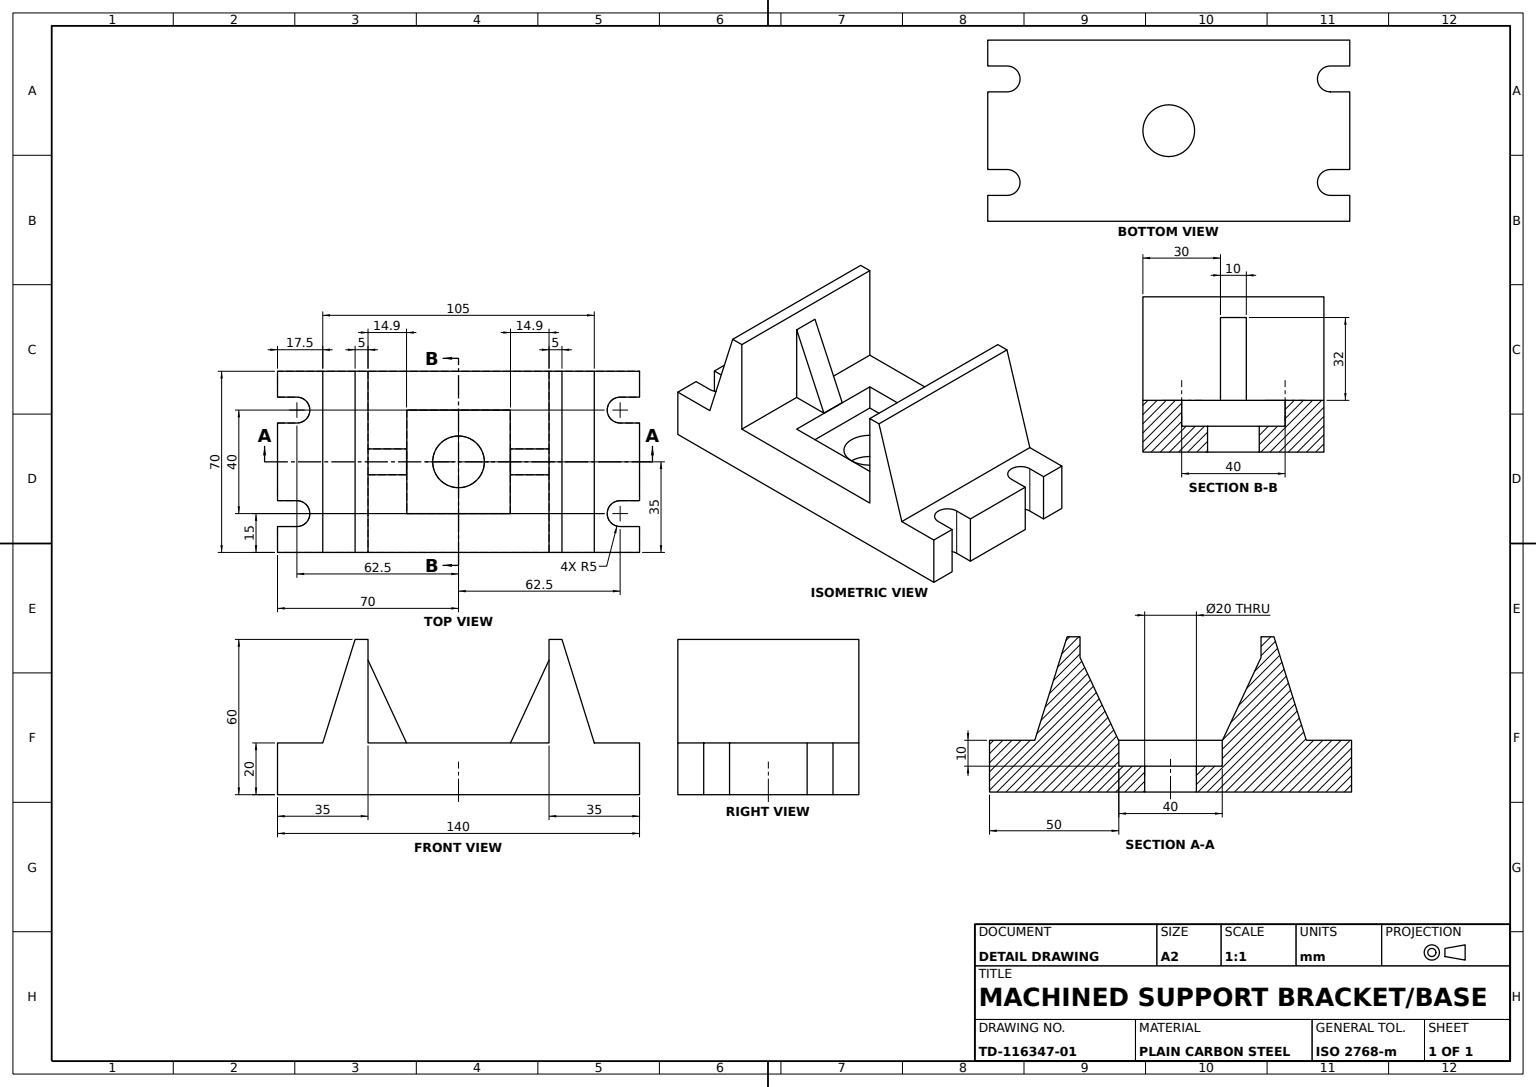
SolidWorks part; units mm, degrees
material "Plain Carbon Steel"
ref_plane "Front Plane" through (0, 0, 0) normal (0, 0, 1) x (1, 0, 0)
ref_plane "Top Plane" through (0, 0, 0) normal (0, 1, 0) x (1, 0, 0)
ref_plane "Right Plane" through (0, 0, 0) normal (1, 0, 0) x (0, 0, -1)
sketch "Base Plate Sketch" plane through (0, 0, 0) normal (0, 1, 0) x (1, 0, 0)
  line L0 (-70, 25) -> (-62.5, 25)
  line L1 (-70, 35) -> (70, 35)
  line L2 (-70, 35) -> (-70, 25)
  line L3 (-70, -35) -> (70, -35)
  line L4 (70, 35) -> (70, 25)
  line L5 (-70, 35) -> (70, -35) construction
  line L6 (-70, -35) -> (70, 35) construction
  line L8 (70, 15) -> (62.5, 15)
  line L9 (-70, -15) -> (-62.5, -15)
  line L11 (70, -25) -> (62.5, -25)
  line L12 (-70, 15) -> (-70, -15)
  line L13 (62.5, 25) -> (70, 25)
  line L14 (-62.5, 15) -> (-70, 15)
  line L15 (70, 15) -> (70, -15)
  line L16 (-70, -25) -> (-70, -35)
  line L17 (62.5, -15) -> (70, -15)
  line L18 (-62.5, -25) -> (-70, -25)
  line L19 (70, -25) -> (70, -35)
  arc A0 (-62.5, -25) -> (-62.5, -15) centre (-62.5, -20) ccw
  arc A1 (-62.5, 15) -> (-62.5, 25) centre (-62.5, 20) ccw
  arc A2 (62.5, 25) -> (62.5, 15) centre (62.5, 20) ccw
  arc A3 (62.5, -15) -> (62.5, -25) centre (62.5, -20) ccw
  point P8 (0, 0)
  dimension "D1" = 20
  dimension "D11" = 10
  dimension "D12" = 10
  dimension "D13" = 10
  dimension "D14" = 10
  dimension "D2" = 20
  dimension "D3" = 20
  dimension "D4" = 20
  dimension "D5" = 62.5
  dimension "D6" = 62.5
  dimension "D7" = 62.5
  dimension "D8" = 62.5
  dimension "D9" = 70
  dimension "D10" = 140
extrude "Base Plate 140x70x20" add sketch "Base Plate Sketch" along normal blind 20
sketch "Centre Hole Sketch" plane through (0, 20, 0) normal (0, 1, 0) x (1, 0, 0)
  circle A0 centre (0, 0) radius 10
  dimension "D1" = 20
extrude "Centre Hole Ø20" cut sketch "Centre Hole Sketch" against normal blind 20
sketch "Centre Pocket Sketch" plane through (0, 20, 0) normal (0, 1, 0) x (1, 0, 0)
  line L1 (-20, 20) -> (20, 20)
  line L2 (-20, 20) -> (-20, -20)
  line L3 (-20, -20) -> (20, -20)
  line L4 (20, 20) -> (20, -20)
  line L5 (-20, 20) -> (20, -20) construction
  line L6 (-20, -20) -> (20, 20) construction
  point P0 (0, 0)
  dimension "D1" = 40
extrude "Centre Pocket 40x40x10" cut sketch "Centre Pocket Sketch" against normal blind 10
sketch "V-Block Uprights Sketch" plane through (0, 0, 35) normal (0, 0, 1) x (1, 0, 0)
  line L0 (-52.5, 20) -> (-35, 20)
  line L1 (-70, 20) -> (70, 20) construction
  line L3 (-70, 20) -> (-70, 0) construction
  line L4 (70, 20) -> (70, 0) construction
  line L6 (35, 20) -> (52.5, 20)
  line L7 (-35, 60) -> (-40, 60)
  line L8 (-40, 60) -> (-52.5, 20)
  line L9 (-35, 20) -> (-35, 60)
  line L10 (35, 60) -> (35, 20)
  line L11 (35, 20) -> (52.5, 20)
  line L12 (35, 60) -> (40, 60)
  line L13 (40, 60) -> (52.5, 20)
  line L14 (35, 20) -> (52.5, 20)
  point P5 (0, 20)
  line M9 (70, 20) -> (-70, 20)
  dimension "D1" = 105
  dimension "D2" = 17.5
  dimension "D3" = 17.5
  dimension "D4" = 70
  dimension "D5" = 40
  dimension "D6" = 17.5
  dimension "D7" = 5
  dimension "D8" = 17.5
  dimension "D9" = 5
extrude "V-Block Uprights" add sketch "V-Block Uprights Sketch" against normal blind 70 contours L9 L7 L8 M9 | L13 L12 L10 M9
ref_plane "Rib Plane" through (0, 0, 0) normal (0, 0, 1) x (1, 0, 0)
sketch "Gusset Rib Sketch" plane through (0, 0, 0) normal (0, 0, 1) x (1, 0, 0)
  line L1 (-35, 20) -> (-35, 60) construction
  line L3 (35, 60) -> (35, 20) construction
  line L4 (-35, 20) -> (-35, 52)
  line L5 (-35, 52) -> (-20.103, 20)
  line L6 (-20.103, 20) -> (-35, 20)
  line L7 (35, 52) -> (35, 20)
  line L8 (35, 52) -> (35, 20)
  line L9 (35, 20) -> (20.1, 20)
  line L10 (-35, 20) -> (35, 20) construction
  line L11 (20.1, 20) -> (35, 52)
  dimension "D1" = 14.897
  dimension "D2" = 32
  dimension "D3" = 32
  dimension "D4" = 14.9
extrude "Gusset Rib" add sketch "Gusset Rib Sketch" along normal mid plane 10 contours L6 L5 L4 | L11 L9 L7
